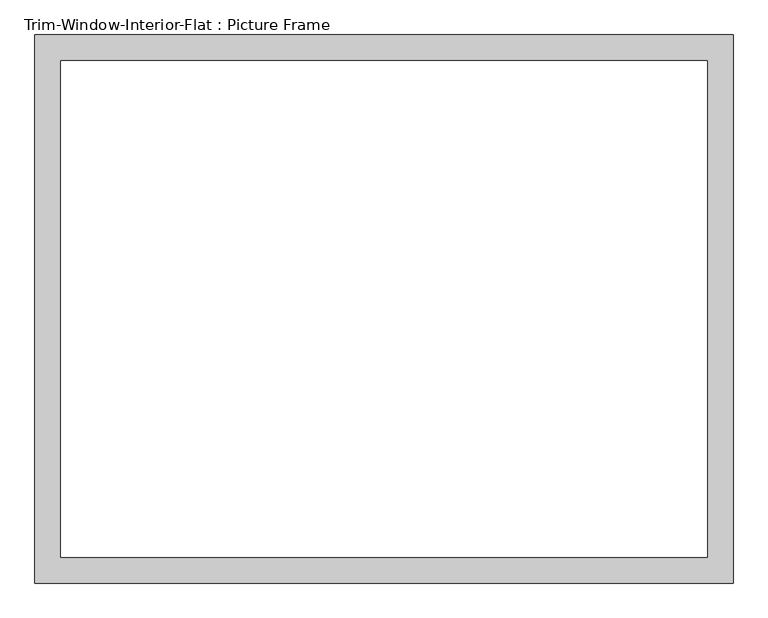
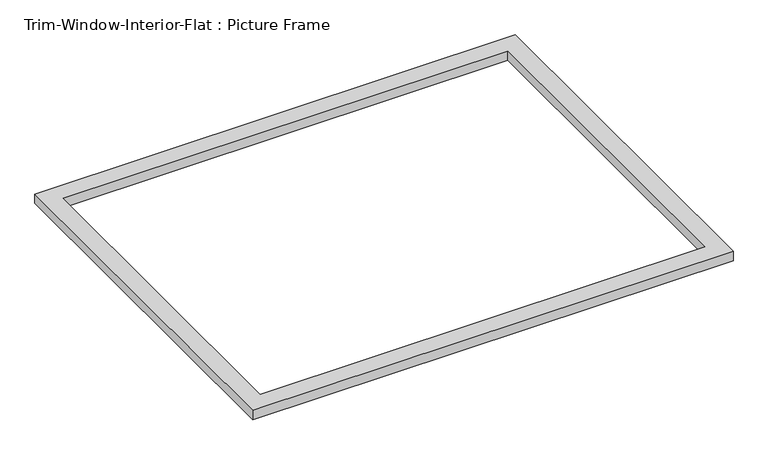
"""IFC4 building model written with IfcOpenShell, lengths in millimetres: proxy geometry, Trim-Window-Interior-Flat : Picture Frame."""

from ifc_helpers import new_model, si_unit, origin, origin_with_axes, place, context, project, spatial, polyline, outline, extrude, source, transform, mapped, element, save


def trim_window_interior_flat_picture_frame_286514af(model_context):
    return source(origin(), model_context, "Body", "SweptSolid", [
        extrude(outline(polyline([(768.35, 44.45), (768.35, -1162.05), (-768.35, -1162.05), (-768.35, 44.45), (768.35, 44.45)]), holes=[polyline([(711.2, -12.7), (-711.2, -12.7), (-711.2, -1104.9), (711.2, -1104.9), (711.2, -12.7)])]), origin_with_axes(), (0.0, 0.0, 1.0), 31.75),
    ])


if __name__ == "__main__":
    model = new_model("IFC4")
    model_context = context("Model", 3, world=origin())
    ifc_project = project(units=[si_unit("LENGTHUNIT", "METRE", prefix="MILLI")], contexts=[model_context])
    site = spatial("IfcSite", under=ifc_project)
    building = spatial("IfcBuilding", under=site)
    placement = place(None, origin())
    trim_window_interior_flat_picture_frame_shape = trim_window_interior_flat_picture_frame_286514af(model_context)
    element("IfcBuildingElementProxy", 1, Name="Trim-Window-Interior-Flat : Picture Frame", ObjectType="Trim-Window-Interior-Flat : Picture Frame", at=placement, inside=building, context=model_context, shape_type="MappedRepresentation", body=[
        mapped(trim_window_interior_flat_picture_frame_shape, transform((0.0, 0.0, 0.0), x_axis=(1.0, 0.0, 0.0), y_axis=(0.0, 1.0, 0.0), z_axis=(0.0, 0.0, 1.0))),
    ])
    save(model, "model.ifc")

# Revit data of these elements
# Type "Trim-Window-Interior-Flat : Picture Frame"
#   Trim Thickness_Picture Frame = 1.25"
#   Trim Width = 2.25"
#   Trim Thickness_with Sill = 0.75"
#   Sill Thickness = 1.25"
#   Opening Width [instance default] = 24"
#   Opening Height [instance default] = 36"
#   Default Elevation = 48"
#   Sill = no
#   Picture Frame = yes
#   Trim Material [instance default] = none
# Element 1 (IfcBuildingElementProxy, "Trim-Window-Interior-Flat : Picture Frame")
#   Opening Width = 57"
#   Opening Height = 44"
#   Trim Material = Wood - Stained
#   Materials on its faces: "Wood - Stained"
# Materials
#   "Wood - Stained": class "Wood", colour RGB 224 178 126, transparency 0, Cost = 0
